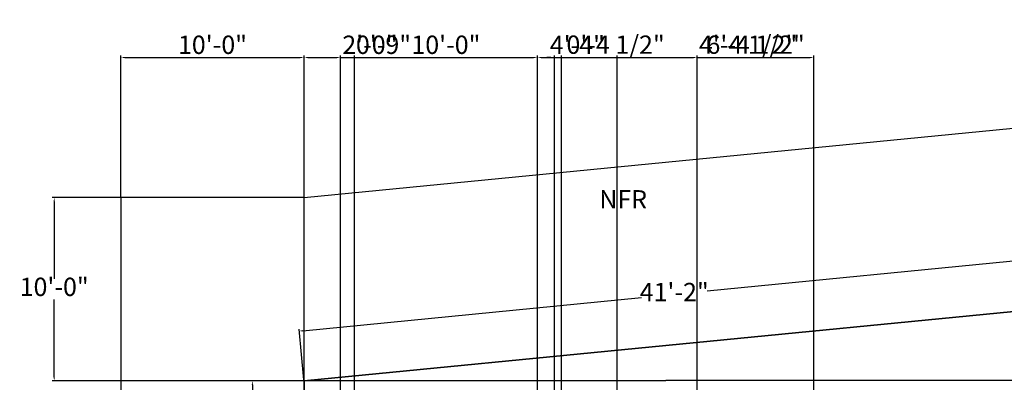
# Model space of a CAD drawing. Units: inches. Extents: x 5307 to 6359, y 4763 to 5474.
# Tile 4 of 5: x 5360 to 6006, y 5237 to 5474. Entities that reach past the tile are written whole.
import ezdxf

# ---------------------------------------------------------------- set-up
doc = ezdxf.new("R2010")
doc.units = ezdxf.units.IN
for name, color, linetype, lineweight in [('A-ANNO-DIMS', 2, 'Continuous', 18), ('A-ANNO-TEXT', 7, 'Continuous', 18), ('C-PROP', 7, 'Continuous', 35), ('ROAD', 240, 'Continuous', 25)]:
    doc.layers.add(name, color=color, linetype=linetype, lineweight=lineweight)
doc.styles.get("Standard").update_dxf_attribs({"font": 'arial.ttf'})
doc.dimstyles.new('ISO-25', dxfattribs={"dimtxt": 12, "dimasz": 2.5, "dimexe": 1.25, "dimexo": 0.625, "dimtad": 1, "dimtih": 1, "dimtoh": 1, "dimlunit": 4, "dimtxsty": 'Standard', "dimcen": 2.5, "dimadec": 0, "dimazin": 0, "dimtfac": 1, "dimtmove": 0, "dimatfit": 3, "dimfxl": 1, "dimarcsym": 0})

# ---------------------------------------------------------------- blocks, each defined once
blk = doc.blocks.new('*D2')
at = {"layer": 'A-ANNO-DIMS', "color": 0, "lineweight": -2, "transparency": 16777216}
for p, q in [((6032.58, 5318.14), (5810.72, 5296.48)), ((6038.19, 5286.41), (6034.95, 5319.62)), ((5545.9, 5270.62), (5767.76, 5292.28)), ((5546.53, 5238.41), (5543.29, 5271.62))]:
    blk.add_line(p, q, dxfattribs=at)
at = {"layer": 'A-ANNO-DIMS', "color": 0, "transparency": 16777216}
for points in [[(6032.54, 5318.55), (6032.62, 5317.72), (6035.07, 5318.38)], [(5545.86, 5271.04), (5545.94, 5270.21), (5543.41, 5270.38)]]:
    blk.add_solid(points, dxfattribs=at)
at = {"layer": 'Defpoints', "color": 0, "transparency": 16777216}
for p in [(6035.07, 5318.38), (6038.25, 5285.78), (5546.59, 5237.78)]:
    blk.add_point(p, dxfattribs=at)
at = {"layer": 'A-ANNO-DIMS', "color": 0, "transparency": 16777216, "insert": (5789.24, 5294.38), "char_height": 12, "attachment_point": 5}
blk.add_mtext('41\'-2"', dxfattribs=at)
blk = doc.blocks.new('*D3')
at = {"layer": 'A-ANNO-DIMS', "color": 0, "lineweight": -2, "transparency": 16777216}
for p, q in [((5545.97, 5237.78), (5511.45, 5237.78)), ((5512.7, 5235.28), (5512.7, 5094.54)), ((5512.7, 4940.28), (5512.7, 5081.03)), ((5545.97, 4937.78), (5511.45, 4937.78))]:
    blk.add_line(p, q, dxfattribs=at)
at = {"layer": 'A-ANNO-DIMS', "color": 0, "transparency": 16777216}
for points in [[(5512.28, 5235.28), (5513.12, 5235.28), (5512.7, 5237.78)], [(5512.28, 4940.28), (5513.12, 4940.28), (5512.7, 4937.78)]]:
    blk.add_solid(points, dxfattribs=at)
at = {"layer": 'Defpoints', "color": 0, "transparency": 16777216}
for p in [(5546.59, 5237.78), (5512.7, 4937.78), (5546.59, 4937.78)]:
    blk.add_point(p, dxfattribs=at)
at = {"layer": 'A-ANNO-DIMS', "color": 0, "transparency": 16777216, "insert": (5512.7, 5087.78), "char_height": 12, "attachment_point": 5}
blk.add_mtext("25'", dxfattribs=at)
blk = doc.blocks.new('*D13')
at = {"layer": 'A-ANNO-DIMS', "color": 0, "lineweight": -2, "transparency": 16777216}
for p, q in [((6038.88, 5405.78), (6325.25, 5405.78)), ((6324, 5403.28), (6324, 5118.54)), ((6324, 4820.28), (6324, 5105.03)), ((5547.22, 4817.78), (6325.25, 4817.78))]:
    blk.add_line(p, q, dxfattribs=at)
at = {"layer": 'A-ANNO-DIMS', "color": 0, "transparency": 16777216}
for points in [[(6323.58, 5403.28), (6324.41, 5403.28), (6324, 5405.78)], [(6323.58, 4820.28), (6324.41, 4820.28), (6324, 4817.78)]]:
    blk.add_solid(points, dxfattribs=at)
at = {"layer": 'Defpoints', "color": 0, "transparency": 16777216}
for p in [(6038.25, 5405.78), (6324, 5405.78), (5546.59, 4817.78)]:
    blk.add_point(p, dxfattribs=at)
at = {"layer": 'A-ANNO-DIMS', "color": 0, "transparency": 16777216, "insert": (6324, 5111.78), "char_height": 12, "attachment_point": 5}
blk.add_mtext('49\'-0"', dxfattribs=at)
blk = doc.blocks.new('*D14')
at = {"layer": 'A-ANNO-DIMS', "color": 0, "lineweight": -2, "transparency": 16777216}
for p, q in [((5546.59, 5238.41), (5546.59, 5450.78)), ((5549.09, 5449.53), (5568.09, 5449.53)), ((5570.59, 5214.43), (5570.59, 5450.78)), ((5570.59, 5449.53), (5606.45, 5449.53))]:
    blk.add_line(p, q, dxfattribs=at)
at = {"layer": 'A-ANNO-DIMS', "color": 0, "transparency": 16777216}
for points in [[(5549.09, 5449.95), (5549.09, 5449.12), (5546.59, 5449.53)], [(5568.09, 5449.95), (5568.09, 5449.12), (5570.59, 5449.53)]]:
    blk.add_solid(points, dxfattribs=at)
at = {"layer": 'Defpoints', "color": 0, "transparency": 16777216}
for p in [(5570.59, 5449.53), (5546.59, 5237.78), (5570.59, 5213.81)]:
    blk.add_point(p, dxfattribs=at)
at = {"layer": 'A-ANNO-DIMS', "color": 0, "transparency": 16777216, "insert": (5589.77, 5456.29), "char_height": 12, "attachment_point": 5}
blk.add_mtext('2\'-0"', dxfattribs=at)
blk = doc.blocks.new('*D16')
at = {"layer": 'A-ANNO-DIMS', "color": 0, "lineweight": -2, "transparency": 16777216}
for p, q in [((5426.59, 5358.41), (5426.59, 5450.78)), ((5429.09, 5449.53), (5544.09, 5449.53)), ((5546.59, 5358.41), (5546.59, 5450.78))]:
    blk.add_line(p, q, dxfattribs=at)
at = {"layer": 'A-ANNO-DIMS', "color": 0, "transparency": 16777216}
for points in [[(5429.09, 5449.95), (5429.09, 5449.12), (5426.59, 5449.53)], [(5544.09, 5449.95), (5544.09, 5449.12), (5546.59, 5449.53)]]:
    blk.add_solid(points, dxfattribs=at)
at = {"layer": 'Defpoints', "color": 0, "transparency": 16777216}
for p in [(5546.59, 5449.53), (5426.59, 5357.78), (5546.59, 5357.78)]:
    blk.add_point(p, dxfattribs=at)
at = {"layer": 'A-ANNO-DIMS', "color": 0, "transparency": 16777216, "insert": (5486.59, 5456.29), "char_height": 12, "attachment_point": 5}
blk.add_mtext('10\'-0"', dxfattribs=at)
blk = doc.blocks.new('*D17')
at = {"layer": 'A-ANNO-DIMS', "color": 0, "lineweight": -2, "transparency": 16777216}
for p, q in [((5545.97, 5357.78), (5381.59, 5357.78)), ((5382.84, 5355.28), (5382.84, 5304.54)), ((5382.84, 5240.28), (5382.84, 5291.03)), ((5545.97, 5237.78), (5381.59, 5237.78))]:
    blk.add_line(p, q, dxfattribs=at)
at = {"layer": 'A-ANNO-DIMS', "color": 0, "transparency": 16777216}
for points in [[(5382.43, 5355.28), (5383.26, 5355.28), (5382.84, 5357.78)], [(5382.43, 5240.28), (5383.26, 5240.28), (5382.84, 5237.78)]]:
    blk.add_solid(points, dxfattribs=at)
at = {"layer": 'Defpoints', "color": 0, "transparency": 16777216}
for p in [(5546.59, 5357.78), (5382.84, 5237.78), (5546.59, 5237.78)]:
    blk.add_point(p, dxfattribs=at)
at = {"layer": 'A-ANNO-DIMS', "color": 0, "transparency": 16777216, "insert": (5382.84, 5297.78), "char_height": 12, "attachment_point": 5}
blk.add_mtext('10\'-0"', dxfattribs=at)
blk = doc.blocks.new('*D19')
at = {"layer": 'A-ANNO-DIMS', "color": 0, "lineweight": -2, "transparency": 16777216}
for p, q in [((5570.59, 5214.43), (5570.59, 5450.78)), ((5573.09, 5449.53), (5577.09, 5449.53)), ((5579.59, 5205.44), (5579.59, 5450.78)), ((5579.59, 5449.53), (5615.24, 5449.53))]:
    blk.add_line(p, q, dxfattribs=at)
at = {"layer": 'A-ANNO-DIMS', "color": 0, "transparency": 16777216}
for points in [[(5573.09, 5449.95), (5573.09, 5449.12), (5570.59, 5449.53)], [(5577.09, 5449.95), (5577.09, 5449.12), (5579.59, 5449.53)]]:
    blk.add_solid(points, dxfattribs=at)
at = {"layer": 'Defpoints', "color": 0, "transparency": 16777216}
for p in [(5579.59, 5449.53), (5570.59, 5213.81), (5579.59, 5204.82)]:
    blk.add_point(p, dxfattribs=at)
at = {"layer": 'A-ANNO-DIMS', "color": 0, "transparency": 16777216, "insert": (5598.67, 5456.29), "char_height": 12, "attachment_point": 5}
blk.add_mtext('0\'-9"', dxfattribs=at)
blk = doc.blocks.new('*D20')
at = {"layer": 'A-ANNO-DIMS', "color": 0, "lineweight": -2, "transparency": 16777216}
for p, q in [((5579.59, 5205.44), (5579.59, 5450.78)), ((5582.09, 5449.53), (5697.09, 5449.53)), ((5699.59, 5205.56), (5699.59, 5450.78))]:
    blk.add_line(p, q, dxfattribs=at)
at = {"layer": 'A-ANNO-DIMS', "color": 0, "transparency": 16777216}
for points in [[(5582.09, 5449.95), (5582.09, 5449.12), (5579.59, 5449.53)], [(5697.09, 5449.95), (5697.09, 5449.12), (5699.59, 5449.53)]]:
    blk.add_solid(points, dxfattribs=at)
at = {"layer": 'Defpoints', "color": 0, "transparency": 16777216}
for p in [(5699.59, 5449.53), (5579.59, 5204.82), (5699.59, 5204.93)]:
    blk.add_point(p, dxfattribs=at)
at = {"layer": 'A-ANNO-DIMS', "color": 0, "transparency": 16777216, "insert": (5639.59, 5456.29), "char_height": 12, "attachment_point": 5}
blk.add_mtext('10\'-0"', dxfattribs=at)
blk = doc.blocks.new('*D21')
at = {"layer": 'A-ANNO-DIMS', "color": 0, "lineweight": -2, "transparency": 16777216}
for p, q in [((5699.59, 5205.56), (5699.59, 5450.78)), ((5702.09, 5449.53), (5749.33, 5449.53)), ((5751.83, 5205.61), (5751.83, 5450.78))]:
    blk.add_line(p, q, dxfattribs=at)
at = {"layer": 'A-ANNO-DIMS', "color": 0, "transparency": 16777216}
for points in [[(5702.09, 5449.95), (5702.09, 5449.12), (5699.59, 5449.53)], [(5749.33, 5449.95), (5749.33, 5449.12), (5751.83, 5449.53)]]:
    blk.add_solid(points, dxfattribs=at)
at = {"layer": 'Defpoints', "color": 0, "transparency": 16777216}
for p in [(5751.83, 5449.53), (5699.59, 5204.93), (5751.83, 5204.98)]:
    blk.add_point(p, dxfattribs=at)
at = {"layer": 'A-ANNO-DIMS', "color": 0, "transparency": 16777216, "insert": (5725.71, 5456.16), "char_height": 12, "attachment_point": 5}
blk.add_mtext('4\'-4"', dxfattribs=at)
blk = doc.blocks.new('*D22')
at = {"layer": 'A-ANNO-DIMS', "color": 0, "lineweight": -2, "transparency": 16777216}
for p, q in [((5751.83, 5205.61), (5751.83, 5450.78)), ((5754.33, 5449.53), (5801.83, 5449.53)), ((5804.33, 5205.66), (5804.33, 5450.78)), ((5804.33, 5449.53), (5868.43, 5449.53))]:
    blk.add_line(p, q, dxfattribs=at)
at = {"layer": 'A-ANNO-DIMS', "color": 0, "transparency": 16777216}
for points in [[(5754.33, 5449.95), (5754.33, 5449.12), (5751.83, 5449.53)], [(5801.83, 5449.95), (5801.83, 5449.12), (5804.33, 5449.53)]]:
    blk.add_solid(points, dxfattribs=at)
at = {"layer": 'Defpoints', "color": 0, "transparency": 16777216}
for p in [(5804.33, 5449.53), (5751.83, 5204.98), (5804.33, 5205.03)]:
    blk.add_point(p, dxfattribs=at)
at = {"layer": 'A-ANNO-DIMS', "color": 0, "transparency": 16777216, "insert": (5837.63, 5456.36), "char_height": 12, "attachment_point": 5}
blk.add_mtext('4\'-4 1/2"', dxfattribs=at)
blk = doc.blocks.new('*D23')
at = {"layer": 'A-ANNO-DIMS', "color": 0, "lineweight": -2, "transparency": 16777216}
for p, q in [((5804.33, 5205.66), (5804.33, 5450.78)), ((5806.83, 5449.53), (5878.33, 5449.53)), ((5880.83, 5205.73), (5880.83, 5450.78))]:
    blk.add_line(p, q, dxfattribs=at)
at = {"layer": 'A-ANNO-DIMS', "color": 0, "transparency": 16777216}
for points in [[(5806.83, 5449.95), (5806.83, 5449.12), (5804.33, 5449.53)], [(5878.33, 5449.95), (5878.33, 5449.12), (5880.83, 5449.53)]]:
    blk.add_solid(points, dxfattribs=at)
at = {"layer": 'Defpoints', "color": 0, "transparency": 16777216}
for p in [(5880.83, 5449.53), (5804.33, 5205.03), (5880.83, 5205.11)]:
    blk.add_point(p, dxfattribs=at)
at = {"layer": 'A-ANNO-DIMS', "color": 0, "transparency": 16777216, "insert": (5842.58, 5456.36), "char_height": 12, "attachment_point": 5}
blk.add_mtext('6\'-4 1/2"', dxfattribs=at)
blk = doc.blocks.new('*D30')
at = {"layer": 'A-ANNO-DIMS', "color": 0, "lineweight": -2, "transparency": 16777216}
for p, q in [((5708.26, 5449.53), (5705.76, 5449.53)), ((5710.76, 4971.41), (5710.76, 5450.78)), ((5710.76, 5449.53), (5715.26, 5449.53)), ((5715.26, 4971.41), (5715.26, 5450.78)), ((5717.76, 5449.53), (5781.37, 5449.53))]:
    blk.add_line(p, q, dxfattribs=at)
at = {"layer": 'A-ANNO-DIMS', "color": 0, "transparency": 16777216}
for points in [[(5708.26, 5449.95), (5708.26, 5449.12), (5710.76, 5449.53)], [(5717.76, 5449.95), (5717.76, 5449.12), (5715.26, 5449.53)]]:
    blk.add_solid(points, dxfattribs=at)
at = {"layer": 'Defpoints', "color": 0, "transparency": 16777216}
for p in [(5715.26, 5449.53), (5710.76, 4970.78), (5715.26, 4970.78)]:
    blk.add_point(p, dxfattribs=at)
at = {"layer": 'A-ANNO-DIMS', "color": 0, "transparency": 16777216, "insert": (5750.81, 5456.36), "char_height": 12, "attachment_point": 5}
blk.add_mtext('0\'-4 1/2"', dxfattribs=at)

msp = doc.modelspace()

# ---------------------------------------------------------------- linework, layer by layer
at = {"layer": 'C-PROP'}
for p, q in [((6038.255, 5285.784), (5546.592, 5237.784)), ((5546.592, 5237.784), (6038.301, 5238.261)), ((5546.592, 5237.784), (5546.592, 4937.784))]:
    msp.add_line(p, q, dxfattribs=at)
at = {"layer": 'ROAD'}
for p, q in [((5546.592, 5357.784), (6038.255, 5405.784)), ((5546.592, 5357.784), (5426.592, 5357.784)), ((5426.592, 5357.784), (5426.592, 4817.784)), ((5546.592, 5237.784), (5546.592, 5357.784))]:
    msp.add_line(p, q, dxfattribs=at)

# ---------------------------------------------------------------- texts
at = {"layer": 'A-ANNO-TEXT', "insert": (5740.124, 5362.645), "char_height": 12, "attachment_point": 1}
msp.add_mtext_dynamic_manual_height_columns('NFR', width=39.8942, gutter_width=12.5, heights=[0], dxfattribs=at)

# ---------------------------------------------------------------- dimensions: what is measured, and where the dimension line sits
at = {"layer": 'A-ANNO-DIMS'}
for base, p1, p2, picture, middle in [((5715.258, 5449.534), (5710.758, 4970.784), (5715.258, 4970.784), '*D30', (5750.814, 5456.363)), ((5804.333, 5449.534), (5751.833, 5204.983), (5804.333, 5205.034), '*D22', (5837.63, 5456.363)), ((5880.833, 5449.534), (5804.333, 5205.034), (5880.833, 5205.108), '*D23', (5842.583, 5456.363)), ((5546.592, 5449.534), (5426.592, 5357.784), (5546.592, 5357.784), '*D16', (5486.592, 5456.286)), ((5570.592, 5449.534), (5546.592, 5237.784), (5570.592, 5213.807), '*D14', (5589.769, 5456.286)), ((5579.592, 5449.534), (5570.592, 5213.807), (5579.592, 5204.816), '*D19', (5598.667, 5456.286)), ((5699.592, 5449.534), (5579.592, 5204.816), (5699.592, 5204.932), '*D20', (5639.592, 5456.286)), ((5751.833, 5449.534), (5699.592, 5204.932), (5751.833, 5204.983), '*D21', (5725.713, 5456.159))]:
    dim = msp.add_linear_dim(base=base, p1=p1, p2=p2, dimstyle='ISO-25', override={"dimdec": 1, "dimlfac": 1, "dimrnd": 0, "dimzin": 1, "dimdsep": 46, "dimlunit": 4, "dimfrac": 2}, dxfattribs=at)
    dim.commit()
    dim.dimension.update_dxf_attribs({"geometry": picture, "text_midpoint": middle})
for base, p1, p2, override, picture, middle in [((6323.996, 5405.784), (5546.592, 4817.784), (6038.255, 5405.784), {"dimdec": 1, "dimlfac": 1, "dimrnd": 0, "dimzin": 1, "dimdsep": 46, "dimlunit": 4, "dimfrac": 2}, '*D13', (6323.996, 5111.784)), ((5382.842, 5237.784), (5546.592, 5357.784), (5546.592, 5237.784), {"dimdec": 1, "dimlfac": 1, "dimrnd": 0, "dimzin": 1, "dimdsep": 46, "dimlunit": 4, "dimfrac": 2}, '*D17', (5382.842, 5297.784)), ((5512.7, 4937.784), (5546.592, 5237.784), (5546.592, 4937.784), {"dimclrd": 0, "dimclre": 0, "dimclrt": 0}, '*D3', (5512.7, 5087.784))]:
    dim = msp.add_linear_dim(base=base, p1=p1, p2=p2, angle=90, dimstyle='ISO-25', override=override, dxfattribs=at)
    dim.commit()
    dim.dimension.update_dxf_attribs({"geometry": picture, "text_midpoint": middle})
dim = msp.add_aligned_dim(p1=(5546.592, 5237.784), p2=(6038.255, 5285.784), distance=32.752, dimstyle='ISO-25', override={"dimclrd": 0, "dimclre": 0, "dimclrt": 0}, dxfattribs=at)
dim.commit()
dim.dimension.update_dxf_attribs({"geometry": '*D2', "text_midpoint": (5789.241, 5294.381)})

doc.saveas('drawing.dxf')
